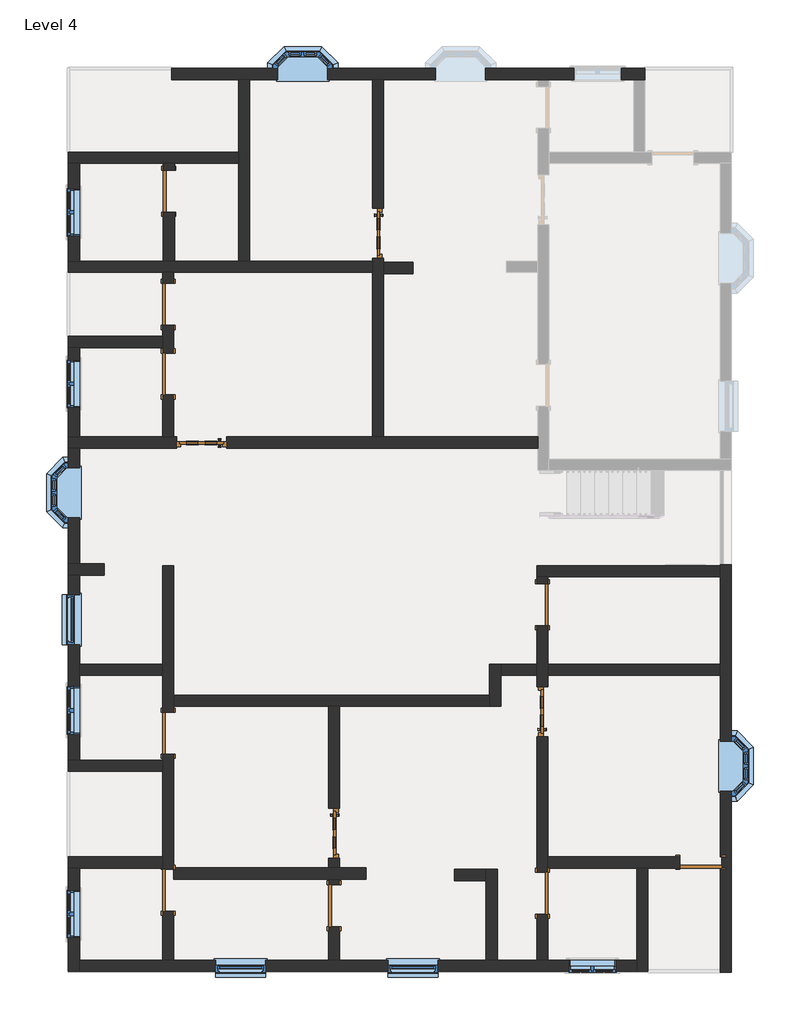
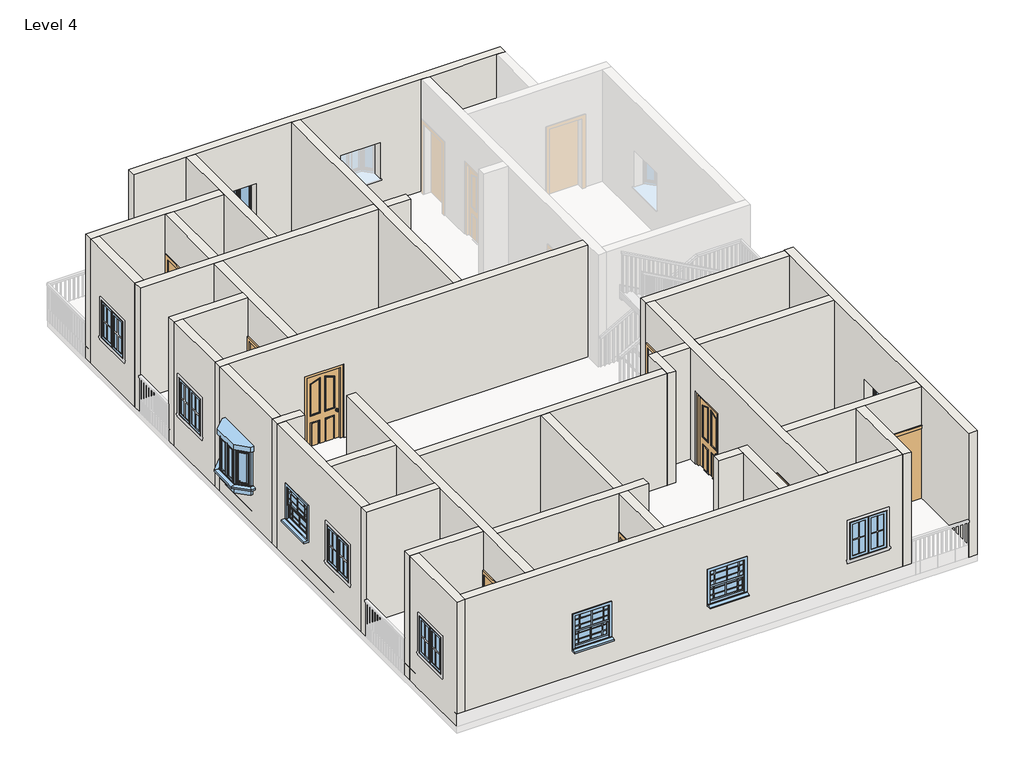
# One storey, part 1 of 4: 34 walls, 13 doors, 11 windows.
# Revit data of these elements (continued)
# Elements 5, 6, 7, 8, 9, 10, 11, 12, 13 (IfcDoor, "Single-Flush : 30\" x 80\"") (continued)
#   Materials on its faces: "Door - Frame", "Door - Panel"
# Elements 14, 23, 24, 25, 28, 31, 32, 33, 34, 35, 36, 37, 38, 39 (IfcWall, "Generic - 4.5\"")
#   Top Offset = 0' - 0"
#   Base Offset = 0' - 0"
#   wall height = 10' - 0"
#   Phase Created = New Construction
#   Base Constraint = Level 4
#   Top Constraint = Level 5
#   Materials on its faces: "Default Wall"
# Elements 15, 20, 26, 30 (IfcWall, "Generic - 4.5\"")
#   Top Offset = 0' - 0"
#   Base Offset = 0' - 0"
#   wall height = 10' - 0"
#   Phase Created = New Construction
#   Base Constraint = Level 4
#   Top Constraint = Level 5
#   Materials on its faces: "Default Wall", "Parking Stripe"
# Elements 16, 17, 18 (IfcWall, "Generic - 4.5\"")
#   Top Offset = 0' - 0"
#   Base Offset = 0' - 0"
#   wall height = 10' - 0"
#   Phase Created = New Construction
#   Base Constraint = Level 4
#   Top Constraint = Level 5
#   Materials on its faces: "Default Wall", "Brick, Soldier Course"
# Elements 19, 21, 22, 29 (IfcWall, "Generic - 4.5\"")
#   Top Offset = 0' - 0"
#   Base Offset = 0' - 0"
#   wall height = 10' - 0"
#   Phase Created = New Construction
#   Base Constraint = Level 4
#   Top Constraint = Level 5
#   Materials on its faces: "Default Wall", "Earth"
# Element 27 (IfcWall, "Generic - 4.5\"")
#   Top Offset = 0' - 0"
#   Base Offset = 0' - 0"
#   wall height = 10' - 0"
#   Phase Created = New Construction
#   Base Constraint = Level 4
#   Top Constraint = Level 5
#   Materials on its faces: "Default Wall", "Parking Stripe", "Cherry"
# Element 40 (IfcWall, "Generic - 9\"")
#   Top Offset = 0' - 0"
#   Base Offset = 0' - 0"
#   wall height = 10' - 0"
#   Phase Created = New Construction
#   Base Constraint = Level 4
#   Top Constraint = Level 5
#   Materials on its faces: "Default Wall", "Door - Panel", "Cherry", "Parking Stripe"
# Element 41 (IfcWall, "Generic - 9\"")
#   Top Offset = 0' - 0"
#   Base Offset = 0' - 0"
#   wall height = 10' - 0"
#   Phase Created = New Construction
#   Base Constraint = Level 4
#   Top Constraint = Level 5
#   Materials on its faces: "Default Wall", "Door - Frame/Mullion", "Parking Stripe"
# Element 42 (IfcWall, "Generic - 9\"")
#   Top Offset = 0' - 0"
#   Base Offset = 0' - 0"
#   wall height = 10' - 0"
#   Phase Created = New Construction
#   Base Constraint = Level 4
#   Top Constraint = Level 5
#   Materials on its faces: "Default Wall", "Parking Stripe"
# Elements 43, 44, 47 (IfcWall, "Generic - 9\"")
#   Top Offset = 0' - 0"
#   Base Offset = 0' - 0"
#   wall height = 10' - 0"
#   Phase Created = New Construction
#   Base Constraint = Level 4
#   Top Constraint = Level 5
#   Materials on its faces: "Default Wall", "Earth"
# Element 45 (IfcWall, "Generic - 9\"")
#   Top Offset = 0' - 0"
#   Base Offset = 0' - 0"
#   wall height = 10' - 0"
#   Phase Created = New Construction
#   Base Constraint = Level 4
#   Top Constraint = Level 5
#   Materials on its faces: "Default Wall", "Parking Stripe", "Cherry"
# Element 46 (IfcWall, "Generic - 9\"")
#   Top Offset = 0' - 0"
#   Base Offset = 0' - 0"
#   wall height = 10' - 0"
#   Phase Created = New Construction
#   Base Constraint = Level 4
#   Top Constraint = Level 5
#   Materials on its faces: "Default Wall", "Cherry"
# Element 48 (IfcWindow, "910x910mm")
#   Mark = "46"
#   Phase Created = New Construction
#   Materials on its faces: "Window Frame", "Glass"
# Element 49 (IfcWindow, "910x910mm")
#   Mark = "49"
#   Phase Created = New Construction
#   Materials on its faces: "Window Frame", "Glass"
# Element 50 (IfcWindow, "910x910mm")
#   Mark = "50"
#   Phase Created = New Construction
#   Materials on its faces: "Window Frame", "Glass"
# Element 51 (IfcWindow, "Window-Casement-Double : 34\" x 36\"")
#   Mark = "55"
#   Window Inset = 0' - 0"
#   Interior Wall Closure = 0' - 2 1/4"
#   Frame Extension = 0' - 0 1/4"
#   Exterior Wall Closure = 0' - 1 1/4"
#   Interior Trim Visibility = yes
#   Exterior Trim Visibility = yes
#   Phase Created = New Construction
#   Materials on its faces: "Wood - Stained", "Glass", "Clad - White"
# Element 52 (IfcWindow, "Window-Casement-Double : 34\" x 36\"")
#   Mark = "56"
#   Window Inset = 0' - 0"
#   Interior Wall Closure = 0' - 2 1/4"
#   Frame Extension = 0' - 0 1/4"
#   Exterior Wall Closure = 0' - 1 1/4"
#   Interior Trim Visibility = yes
#   Exterior Trim Visibility = yes
#   Phase Created = New Construction
#   Materials on its faces: "Wood - Stained", "Glass", "Clad - White"
# Element 53 (IfcWindow, "Window-Casement-Double : 34\" x 36\"")
#   Mark = "58"
#   Window Inset = 0' - 0"
#   Interior Wall Closure = 0' - 2 1/4"
#   Frame Extension = 0' - 0 1/4"
#   Exterior Wall Closure = 0' - 1 1/4"
#   Interior Trim Visibility = yes
#   Exterior Trim Visibility = yes
#   Phase Created = New Construction
#   Materials on its faces: "Wood - Stained", "Glass", "Clad - White"
# Element 54 (IfcWindow, "Window-Casement-Double : 34\" x 36\"")
#   Mark = "59"
#   Window Inset = 0' - 0"
#   Interior Wall Closure = 0' - 2 1/4"
#   Frame Extension = 0' - 0 1/4"
#   Exterior Wall Closure = 0' - 1 1/4"
#   Interior Trim Visibility = yes
#   Exterior Trim Visibility = yes
#   Phase Created = New Construction
#   Materials on its faces: "Wood - Stained", "Glass", "Clad - White"
# Element 55 (IfcWindow, "Window-Casement-Double : 34\" x 36\"")
#   Mark = "60"
#   Window Inset = 0' - 0"
#   Interior Wall Closure = 0' - 2 1/4"
#   Frame Extension = 0' - 0 1/4"
#   Exterior Wall Closure = 0' - 1 1/4"
#   Interior Trim Visibility = yes
#   Exterior Trim Visibility = yes
#   Phase Created = New Construction
#   Materials on its faces: "Wood - Stained", "Glass", "Clad - White"
# Element 56 (IfcWindow, "Windows_Sash_w-Bars_1 : 910x910mm")
#   Mark = "51"
#   Phase Created = New Construction
#   Materials on its faces: "Window Frame", "Glass"
# Element 57 (IfcWindow, "Windows_Sash_w-Bars_1 : 910x910mm")
#   Mark = "52"
#   Phase Created = New Construction
#   Materials on its faces: "Window Frame", "Glass"
# Element 58 (IfcWindow, "Windows_Sash_w-Bars_1 : 910x910mm")
#   Mark = "53"
#   Phase Created = New Construction
#   Materials on its faces: "Window Frame", "Glass"
# Materials
#   "Door - Glazing": colour RGB 0 0 255, transparency 0.75
#   "Door - Panel": class "Wood", colour RGB 210 159 95, transparency 0, Cost = 0
#   "Door - Frame/Mullion": class "Wood", colour RGB 212 179 113, transparency 0
#   "Door - Handle": colour RGB 247 247 247, transparency 0
#   "Door - Frame": colour RGB 118 70 51, transparency 0, Cost = 0
#   "Window Frame": colour RGB 249 249 249, transparency 0
#   "Glass": class "Glass", colour RGB 0 128 192, transparency 0.75, Description = "Soda Lime Glass", Cost = 0
#   "Wood - Stained": class "Wood", colour RGB 224 178 126, transparency 0, Cost = 0
#   "Clad - White": class "Wood", colour RGB 242 242 238, transparency 0, Cost = 0
#   "Default Wall": colour RGB 128 128 128, transparency 0, Cost = 0
#   "Parking Stripe": class "Paint", colour RGB 250 250 91, transparency 0, Cost = 0
#   "Brick, Soldier Course": class "Masonry", colour RGB 170 98 104, transparency 0, Description = "Common brick soldier coursed", Cost = 0
#   "Earth": class "Generic", colour RGB 97 75 62, transparency 0, Description = "Soil", Cost = 0
#   "Cherry": class "Wood", colour RGB 226 177 128, transparency 0, Description = "Prunus Serotina", Cost = 0
